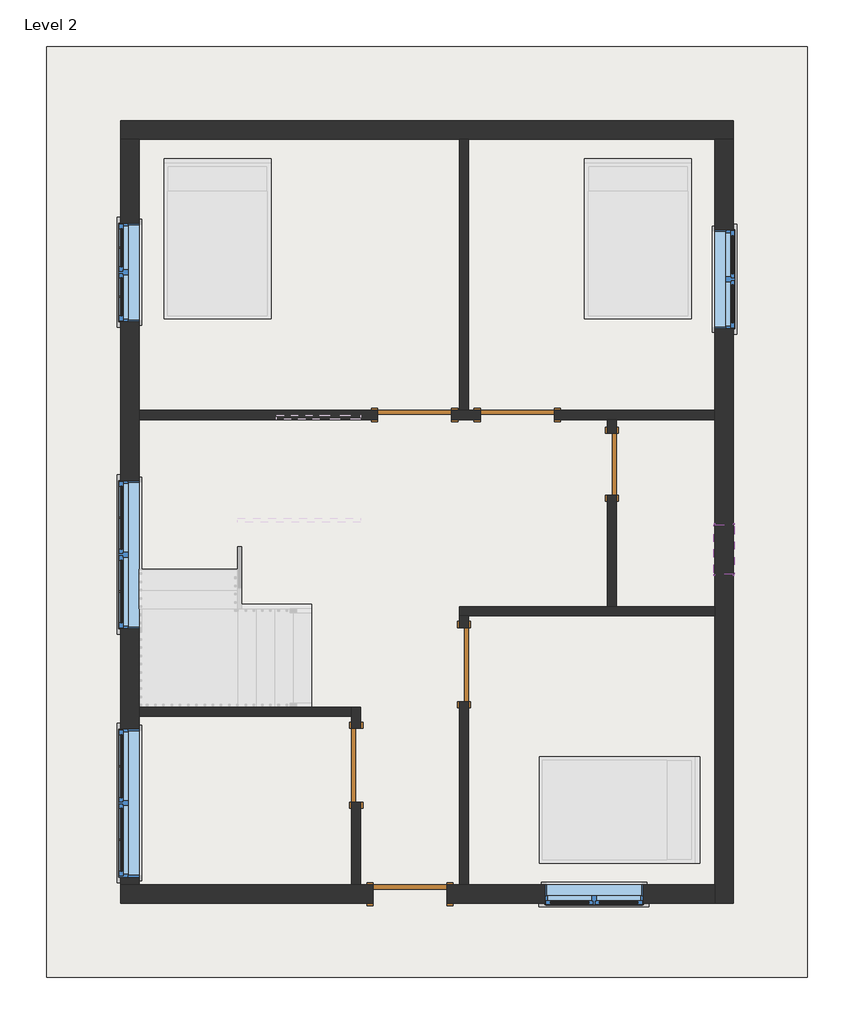
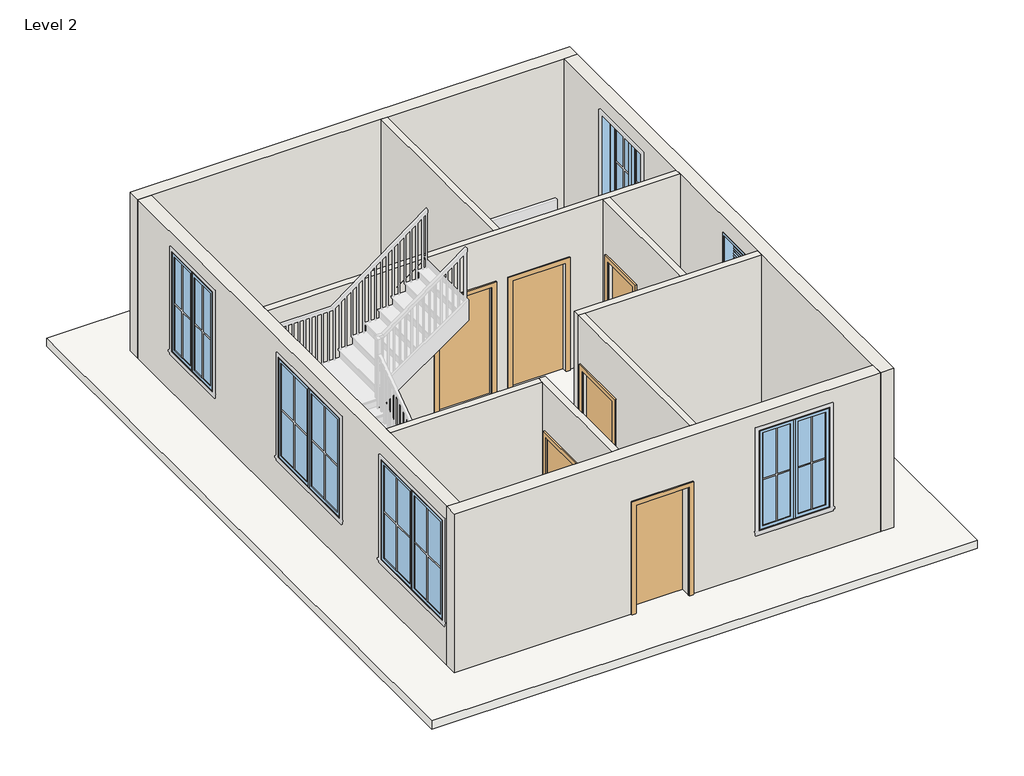
# One storey, part 1 of 3: 11 walls, 6 doors, 6 windows, 1 roof.
"""IFC4 building model written with IfcOpenShell, lengths in millimetres."""

from ifc_helpers import new_model, si_unit, frame, origin, place, context, project, spatial, polyline, outline, extrude, faceted_brep, transform, mapped, element, save
from components import door_f2b275c1, single_flush_door_3_e5f9f3c4, single_flush_door_3_305aa2a5, single_flush_door_3_a90ba1ad, window_casement_double_win_4_6ca1769e, window_casement_double_win_6_ce442eab, window_f2d8fef0

model = new_model("IFC4")

# Units and contexts
model_context = context("Model", 3, world=origin())
ifc_project = project(units=[si_unit("LENGTHUNIT", "METRE", prefix="MILLI")], contexts=[model_context])

# Site, building, storey
site = spatial("IfcSite", under=ifc_project)
building = spatial("IfcBuilding", under=site)
storey = spatial("IfcBuildingStorey", under=building, Name="Level 2", Elevation=3048.0)

# Doors
placement = place(None, origin())
door_shape = door_f2b275c1(model_context)
element("IfcDoor", 1, ObjectType="Single-Flush : 2'6\"", at=placement, inside=storey, context=model_context, shape_type="MappedRepresentation", body=[
    mapped(door_shape, transform((1031.6394609, 262.5126239, 3048.0), x_axis=(0.0, 1.0, 0.0), y_axis=(-1.0, 0.0, 0.0), z_axis=(0.0, 0.0, 1.0))),
])
single_flush_door_3_shape = single_flush_door_3_e5f9f3c4(model_context)
element("IfcDoor", 2, ObjectType="Single-Flush : door 3'", at=placement, inside=storey, context=model_context, shape_type="MappedRepresentation", body=[
    mapped(single_flush_door_3_shape, transform((-1406.7605391, 872.1126239, 3048.0), x_axis=(1.0, 0.0, 0.0), y_axis=(0.0, 1.0, 0.0), z_axis=(0.0, 0.0, 1.0))),
])
element("IfcDoor", 3, ObjectType="Single-Flush : door 3'", at=placement, inside=storey, context=model_context, shape_type="MappedRepresentation", body=[
    mapped(single_flush_door_3_shape, transform((-2130.6605391, -3458.5873761, 3048.0), x_axis=(0.0, 1.0, 0.0), y_axis=(-1.0, 0.0, 0.0), z_axis=(0.0, 0.0, 1.0))),
])
single_flush_door_3_2_shape = single_flush_door_3_305aa2a5(model_context)
element("IfcDoor", 4, ObjectType="Single-Flush : door 3'", at=placement, inside=storey, context=model_context, shape_type="MappedRepresentation", body=[
    mapped(single_flush_door_3_2_shape, transform((-136.7605391, 872.1126239, 3048.0), x_axis=(-1.0, 0.0, 0.0), y_axis=(0.0, -1.0, 0.0), z_axis=(0.0, 0.0, 1.0))),
])
element("IfcDoor", 5, ObjectType="Single-Flush : door 3'", at=placement, inside=storey, context=model_context, shape_type="MappedRepresentation", body=[
    mapped(single_flush_door_3_2_shape, transform((-797.1605391, -2213.9873761, 3048.0), x_axis=(0.0, 1.0, 0.0), y_axis=(-1.0, 0.0, 0.0), z_axis=(0.0, 0.0, 1.0))),
])
single_flush_door_3_3_shape = single_flush_door_3_a90ba1ad(model_context)
element("IfcDoor", 6, ObjectType="Single-Flush : door 3'", at=placement, inside=storey, context=model_context, shape_type="MappedRepresentation", body=[
    mapped(single_flush_door_3_3_shape, transform((-1463.9105391, -5052.4373761, 3048.0), x_axis=(-1.0, 0.0, 0.0), y_axis=(0.0, -1.0, 0.0), z_axis=(0.0, 0.0, 1.0))),
])

# Roof
element("IfcRoof", 7, ObjectType="Generic - 12\"", at=placement, inside=storey, context=model_context, shape_type="SweptSolid", body=[
    extrude(outline(polyline([(-5959.7105391, 5425.0626239), (3450.9894609, 5425.0626239), (3450.9894609, -6081.1373761), (-5959.7105391, -6081.1373761), (-5959.7105391, 5425.0626239)])), frame((0.0, 0.0, 3048.0), z_axis=(0.0, 0.0, 1.0), x_axis=(1.0, 0.0, 0.0)), (0.0, 0.0, 1.0), 152.4),
])

# Walls
element("IfcWall", 8, ObjectType="WALL 4.5\"", at=placement, inside=storey, context=model_context, shape_type="SweptSolid", body=[
    extrude(outline(polyline([(-854.3105391, 929.2626239), (-854.3105391, 4282.0626239), (-740.0105391, 4282.0626239), (-740.0105391, 929.2626239), (-854.3105391, 929.2626239)])), frame((0.0, 0.0, 3048.0), z_axis=(0.0, 0.0, 1.0), x_axis=(1.0, 0.0, 0.0)), (0.0, 0.0, 1.0), 3048.0),
])
element("IfcWall", 9, ObjectType="WALL 4.5\"", at=placement, inside=storey, context=model_context, shape_type="Brep", body=[
    faceted_brep([(-949.5605391, 814.9626239, 3048.0), (-593.9605391, 814.9626239, 3048.0), (-593.9605391, 814.9626239, 5181.6), (320.4394609, 814.9626239, 5181.6), (320.4394609, 814.9626239, 3048.0), (974.4894609, 814.9626239, 3048.0), (1088.7894609, 814.9626239, 3048.0), (2307.9894609, 814.9626239, 3048.0), (2307.9894609, 814.9626239, 6096.0), (1088.7894609, 814.9626239, 6096.0), (974.4894609, 814.9626239, 6096.0), (-4816.7105391, 814.9626239, 6096.0), (-4816.7105391, 814.9626239, 3048.0), (-1863.9605391, 814.9626239, 3048.0), (-1863.9605391, 814.9626239, 5181.6), (-949.5605391, 814.9626239, 5181.6), (-593.9605391, 929.2626239, 5181.6), (-593.9605391, 929.2626239, 3048.0), (-740.0105391, 929.2626239, 3048.0), (-854.3105391, 929.2626239, 3048.0), (-949.5605391, 929.2626239, 3048.0), (-949.5605391, 929.2626239, 5181.6), (-1863.9605391, 929.2626239, 5181.6), (-1863.9605391, 929.2626239, 3048.0), (-4816.7105391, 929.2626239, 3048.0), (-4816.7105391, 929.2626239, 6096.0), (-854.3105391, 929.2626239, 6096.0), (-740.0105391, 929.2626239, 6096.0), (2307.9894609, 929.2626239, 6096.0), (2307.9894609, 929.2626239, 3048.0), (320.4394609, 929.2626239, 3048.0), (320.4394609, 929.2626239, 5181.6)], [[[0, 1, 2, 3, 4, 5, 6, 7, 8, 9, 10, 11, 12, 13, 14, 15]], [[16, 17, 18, 19, 20, 21, 22, 23, 24, 25, 26, 27, 28, 29, 30, 31]], [[13, 12, 24, 23]], [[30, 29, 7, 6, 5, 4]], [[20, 19, 18, 17, 1, 0]], [[8, 7, 29, 28]], [[12, 11, 25, 24]], [[21, 20, 0, 15]], [[22, 21, 15, 14]], [[23, 22, 14, 13]], [[2, 1, 17, 16]], [[3, 2, 16, 31]], [[4, 3, 31, 30]], [[11, 10, 9, 8, 28, 27, 26, 25]]]),
])
element("IfcWall", 10, ObjectType="WALL 4.5\"", at=placement, inside=storey, context=model_context, shape_type="SweptSolid", body=[
    extrude(outline(polyline([(814.9626239, 3048.0), (643.5126239, 3048.0), (643.5126239, 5080.0), (-118.4873761, 5080.0), (-118.4873761, 3048.0), (-1496.4373761, 3048.0), (-1496.4373761, 6096.0), (814.9626239, 6096.0), (814.9626239, 3048.0)])), frame((974.4894609, 0.0, 0.0), z_axis=(1.0, 0.0, 0.0), x_axis=(0.0, 1.0, 0.0)), (0.0, 0.0, 1.0), 114.3),
])
element("IfcWall", 11, ObjectType="WALL 4.5\"", at=placement, inside=storey, context=model_context, shape_type="Brep", body=[
    faceted_brep([(2307.9894609, -1496.4373761, 3048.0), (1088.7894609, -1496.4373761, 3048.0), (974.4894609, -1496.4373761, 3048.0), (-854.3105391, -1496.4373761, 3048.0), (-854.3105391, -1496.4373761, 6096.0), (974.4894609, -1496.4373761, 6096.0), (1088.7894609, -1496.4373761, 6096.0), (2307.9894609, -1496.4373761, 6096.0), (2307.9894609, -1610.7373761, 3048.0), (2307.9894609, -1610.7373761, 6096.0), (-740.0105391, -1610.7373761, 6096.0), (-854.3105391, -1610.7373761, 6096.0), (-854.3105391, -1610.7373761, 3048.0), (-740.0105391, -1610.7373761, 3048.0)], [[[0, 1, 2, 3, 4, 5, 6, 7]], [[8, 9, 10, 11, 12, 13]], [[3, 2, 1, 0, 8, 13, 12]], [[0, 7, 9, 8]], [[4, 3, 12, 11]], [[7, 6, 5, 4, 11, 10, 9]]]),
])
element("IfcWall", 12, ObjectType="WALL 4.5\"", at=placement, inside=storey, context=model_context, shape_type="SweptSolid", body=[
    extrude(outline(polyline([(-1610.7373761, 3048.0), (-1756.7873761, 3048.0), (-1756.7873761, 5181.6), (-2671.1873761, 5181.6), (-2671.1873761, 3048.0), (-4938.1373761, 3048.0), (-4938.1373761, 6096.0), (-1610.7373761, 6096.0), (-1610.7373761, 3048.0)])), frame((-854.3105391, 0.0, 0.0), z_axis=(1.0, 0.0, 0.0), x_axis=(0.0, 1.0, 0.0)), (0.0, 0.0, 1.0), 114.3),
])
element("IfcWall", 13, ObjectType="WALL 4.5\"", at=placement, inside=storey, context=model_context, shape_type="Brep", body=[
    faceted_brep([(-2073.5105391, -3001.3873761, 5181.6), (-2073.5105391, -3001.3873761, 3048.0), (-2073.5105391, -2741.0373761, 3048.0), (-2073.5105391, -2741.0373761, 6096.0), (-2073.5105391, -4938.1373761, 6096.0), (-2073.5105391, -4938.1373761, 3048.0), (-2073.5105391, -3915.7873761, 3048.0), (-2073.5105391, -3915.7873761, 5181.6), (-2187.8105391, -2741.0373761, 3048.0), (-2187.8105391, -2855.3373761, 3048.0), (-2187.8105391, -3001.3873761, 3048.0), (-2187.8105391, -3001.3873761, 5181.6), (-2187.8105391, -3915.7873761, 5181.6), (-2187.8105391, -3915.7873761, 3048.0), (-2187.8105391, -4938.1373761, 3048.0), (-2187.8105391, -4938.1373761, 6096.0), (-2187.8105391, -2855.3373761, 6096.0), (-2187.8105391, -2741.0373761, 6096.0)], [[[0, 1, 2, 3, 4, 5, 6, 7]], [[8, 9, 10, 11, 12, 13, 14, 15, 16, 17]], [[6, 5, 14, 13]], [[2, 1, 10, 9, 8]], [[5, 4, 15, 14]], [[3, 2, 8, 17]], [[11, 10, 1, 0]], [[12, 11, 0, 7]], [[13, 12, 7, 6]], [[4, 3, 17, 16, 15]]]),
])
element("IfcWall", 14, ObjectType="WALL 4.5\"", at=placement, inside=storey, context=model_context, shape_type="SweptSolid", body=[
    extrude(outline(polyline([(-4816.7105391, -2741.0373761), (-2187.8105391, -2741.0373761), (-2187.8105391, -2855.3373761), (-4816.7105391, -2855.3373761), (-4816.7105391, -2741.0373761)])), frame((0.0, 0.0, 3048.0), z_axis=(0.0, 0.0, 1.0), x_axis=(1.0, 0.0, 0.0)), (0.0, 0.0, 1.0), 3048.0),
])
element("IfcWall", 15, ObjectType="WALL 9\"", at=placement, inside=storey, context=model_context, shape_type="Brep", body=[
    faceted_brep([(-5045.3105391, 4282.0626239, 3048.0), (-4816.7105391, 4282.0626239, 3048.0), (-854.3105391, 4282.0626239, 3048.0), (-740.0105391, 4282.0626239, 3048.0), (2307.9894609, 4282.0626239, 3048.0), (2536.5894609, 4282.0626239, 3048.0), (2536.5894609, 4282.0626239, 6096.0), (2307.9894609, 4282.0626239, 6096.0), (-740.0105391, 4282.0626239, 6096.0), (-854.3105391, 4282.0626239, 6096.0), (-4816.7105391, 4282.0626239, 6096.0), (-5045.3105391, 4282.0626239, 6096.0), (-5045.3105391, 4510.6626239, 3048.0), (-5045.3105391, 4510.6626239, 6096.0), (2536.5894609, 4510.6626239, 6096.0), (2536.5894609, 4510.6626239, 3048.0)], [[[0, 1, 2, 3, 4, 5, 6, 7, 8, 9, 10, 11]], [[12, 13, 14, 15]], [[5, 4, 3, 2, 1, 0, 12, 15]], [[6, 5, 15, 14]], [[0, 11, 13, 12]], [[11, 10, 9, 8, 7, 6, 14, 13]]]),
])
element("IfcWall", 16, ObjectType="WALL 9\"", at=placement, inside=storey, context=model_context, shape_type="Brep", body=[
    faceted_brep([(2307.9894609, 4282.0626239, 3048.0), (2307.9894609, 929.2626239, 3048.0), (2307.9894609, 814.9626239, 3048.0), (2307.9894609, -1496.4373761, 3048.0), (2307.9894609, -1610.7373761, 3048.0), (2307.9894609, -4938.1373761, 3048.0), (2307.9894609, -5166.7373761, 3048.0), (2307.9894609, -5166.7373761, 6096.0), (2307.9894609, -4938.1373761, 6096.0), (2307.9894609, -1610.7373761, 6096.0), (2307.9894609, -1496.4373761, 6096.0), (2307.9894609, 814.9626239, 6096.0), (2307.9894609, 929.2626239, 6096.0), (2307.9894609, 4282.0626239, 6096.0), (2307.9894609, 1938.9126239, 5791.2), (2307.9894609, 1938.9126239, 3962.4), (2307.9894609, 3158.1126239, 3962.4), (2307.9894609, 3158.1126239, 5791.2), (2307.9894609, -486.7873761, 5791.2), (2307.9894609, -1096.3873761, 5791.2), (2307.9894609, -1096.3873761, 5181.6), (2307.9894609, -486.7873761, 5181.6), (2536.5894609, 4282.0626239, 3048.0), (2536.5894609, 4282.0626239, 6096.0), (2536.5894609, -5166.7373761, 6096.0), (2536.5894609, -5166.7373761, 3048.0), (2536.5894609, 1938.9126239, 5791.2), (2536.5894609, 3158.1126239, 5791.2), (2536.5894609, 3158.1126239, 3962.4), (2536.5894609, 1938.9126239, 3962.4), (2536.5894609, -486.7873761, 5791.2), (2536.5894609, -486.7873761, 5181.6), (2536.5894609, -1096.3873761, 5181.6), (2536.5894609, -1096.3873761, 5791.2)], [[[0, 1, 2, 3, 4, 5, 6, 7, 8, 9, 10, 11, 12, 13], [14, 15, 16, 17], [18, 19, 20, 21]], [[22, 23, 24, 25], [26, 27, 28, 29], [30, 31, 32, 33]], [[6, 5, 4, 3, 2, 1, 0, 22, 25]], [[0, 13, 23, 22]], [[7, 6, 25, 24]], [[15, 14, 26, 29]], [[16, 15, 29, 28]], [[17, 16, 28, 27]], [[14, 17, 27, 26]], [[31, 30, 18, 21]], [[32, 31, 21, 20]], [[33, 32, 20, 19]], [[30, 33, 19, 18]], [[13, 12, 11, 10, 9, 8, 7, 24, 23]]]),
])
element("IfcWall", 17, ObjectType="WALL 9\"", at=placement, inside=storey, context=model_context, shape_type="Brep", body=[
    faceted_brep([(-1921.1105391, -4938.1373761, 5181.6), (-1921.1105391, -4938.1373761, 3048.0), (-2073.5105391, -4938.1373761, 3048.0), (-2187.8105391, -4938.1373761, 3048.0), (-4816.7105391, -4938.1373761, 3048.0), (-5045.3105391, -4938.1373761, 3048.0), (-5045.3105391, -4938.1373761, 6096.0), (-4816.7105391, -4938.1373761, 6096.0), (-2187.8105391, -4938.1373761, 6096.0), (-2073.5105391, -4938.1373761, 6096.0), (-854.3105391, -4938.1373761, 6096.0), (-740.0105391, -4938.1373761, 6096.0), (2307.9894609, -4938.1373761, 6096.0), (2307.9894609, -4938.1373761, 3048.0), (-740.0105391, -4938.1373761, 3048.0), (-854.3105391, -4938.1373761, 3048.0), (-1006.7105391, -4938.1373761, 3048.0), (-1006.7105391, -4938.1373761, 5181.6), (202.9644609, -4938.1373761, 5791.2), (202.9644609, -4938.1373761, 3962.4), (1422.1644609, -4938.1373761, 3962.4), (1422.1644609, -4938.1373761, 5791.2), (-5045.3105391, -5166.7373761, 3048.0), (-1921.1105391, -5166.7373761, 3048.0), (-1921.1105391, -5166.7373761, 5181.6), (-1006.7105391, -5166.7373761, 5181.6), (-1006.7105391, -5166.7373761, 3048.0), (2307.9894609, -5166.7373761, 3048.0), (2307.9894609, -5166.7373761, 6096.0), (-5045.3105391, -5166.7373761, 6096.0), (202.9644609, -5166.7373761, 5791.2), (1422.1644609, -5166.7373761, 5791.2), (1422.1644609, -5166.7373761, 3962.4), (202.9644609, -5166.7373761, 3962.4)], [[[0, 1, 2, 3, 4, 5, 6, 7, 8, 9, 10, 11, 12, 13, 14, 15, 16, 17], [18, 19, 20, 21]], [[22, 23, 24, 25, 26, 27, 28, 29], [30, 31, 32, 33]], [[5, 4, 3, 2, 1, 23, 22]], [[16, 15, 14, 13, 27, 26]], [[13, 12, 28, 27]], [[6, 5, 22, 29]], [[19, 18, 30, 33]], [[20, 19, 33, 32]], [[21, 20, 32, 31]], [[18, 21, 31, 30]], [[24, 23, 1, 0]], [[25, 24, 0, 17]], [[26, 25, 17, 16]], [[12, 11, 10, 9, 8, 7, 6, 29, 28]]]),
])
element("IfcWall", 18, ObjectType="WALL 9\"", at=placement, inside=storey, context=model_context, shape_type="Brep", body=[
    faceted_brep([(-4816.7105391, -4938.1373761, 3048.0), (-4816.7105391, -2855.3373761, 3048.0), (-4816.7105391, -2741.0373761, 3048.0), (-4816.7105391, 814.9626239, 3048.0), (-4816.7105391, 929.2626239, 3048.0), (-4816.7105391, 4282.0626239, 3048.0), (-4816.7105391, 4282.0626239, 6096.0), (-4816.7105391, 929.2626239, 6096.0), (-4816.7105391, 814.9626239, 6096.0), (-4816.7105391, -2741.0373761, 6096.0), (-4816.7105391, -2855.3373761, 6096.0), (-4816.7105391, -4938.1373761, 6096.0), (-4816.7105391, -3010.9123761, 5791.2), (-4816.7105391, -3010.9123761, 3962.4), (-4816.7105391, -4839.7123761, 3962.4), (-4816.7105391, -4839.7123761, 5791.2), (-4816.7105391, 59.3126239, 5791.2), (-4816.7105391, 59.3126239, 3962.4), (-4816.7105391, -1769.4873761, 3962.4), (-4816.7105391, -1769.4873761, 5791.2), (-4816.7105391, 3243.8376239, 5791.2), (-4816.7105391, 3243.8376239, 3962.4), (-4816.7105391, 2024.6376239, 3962.4), (-4816.7105391, 2024.6376239, 5791.2), (-5045.3105391, -4938.1373761, 3048.0), (-5045.3105391, -4938.1373761, 6096.0), (-5045.3105391, 4282.0626239, 6096.0), (-5045.3105391, 4282.0626239, 3048.0), (-5045.3105391, -3010.9123761, 5791.2), (-5045.3105391, -4839.7123761, 5791.2), (-5045.3105391, -4839.7123761, 3962.4), (-5045.3105391, -3010.9123761, 3962.4), (-5045.3105391, 59.3126239, 5791.2), (-5045.3105391, -1769.4873761, 5791.2), (-5045.3105391, -1769.4873761, 3962.4), (-5045.3105391, 59.3126239, 3962.4), (-5045.3105391, 3243.8376239, 5791.2), (-5045.3105391, 2024.6376239, 5791.2), (-5045.3105391, 2024.6376239, 3962.4), (-5045.3105391, 3243.8376239, 3962.4)], [[[0, 1, 2, 3, 4, 5, 6, 7, 8, 9, 10, 11], [12, 13, 14, 15], [16, 17, 18, 19], [20, 21, 22, 23]], [[24, 25, 26, 27], [28, 29, 30, 31], [32, 33, 34, 35], [36, 37, 38, 39]], [[5, 4, 3, 2, 1, 0, 24, 27]], [[6, 5, 27, 26]], [[0, 11, 25, 24]], [[13, 12, 28, 31]], [[14, 13, 31, 30]], [[15, 14, 30, 29]], [[12, 15, 29, 28]], [[17, 16, 32, 35]], [[18, 17, 35, 34]], [[19, 18, 34, 33]], [[16, 19, 33, 32]], [[21, 20, 36, 39]], [[22, 21, 39, 38]], [[23, 22, 38, 37]], [[20, 23, 37, 36]], [[11, 10, 9, 8, 7, 6, 26, 25]]]),
])

# Windows
window_casement_double_win_4_shape = window_casement_double_win_4_6ca1769e(model_context)
element("IfcWindow", 19, ObjectType="Window-Casement-Double : win 4'", at=placement, inside=storey, context=model_context, shape_type="MappedRepresentation", body=[
    mapped(window_casement_double_win_4_shape, transform((812.5644609, -5052.4373761, 3048.0), x_axis=(-1.0, 0.0, 0.0), y_axis=(0.0, -1.0, 0.0), z_axis=(0.0, 0.0, 1.0))),
])
element("IfcWindow", 20, ObjectType="Window-Casement-Double : win 4'", at=placement, inside=storey, context=model_context, shape_type="MappedRepresentation", body=[
    mapped(window_casement_double_win_4_shape, transform((2422.2894609, 2548.5126239, 3048.0), x_axis=(0.0, -1.0, 0.0), y_axis=(1.0, 0.0, 0.0), z_axis=(0.0, 0.0, 1.0))),
])
element("IfcWindow", 21, ObjectType="Window-Casement-Double : win 4'", at=placement, inside=storey, context=model_context, shape_type="MappedRepresentation", body=[
    mapped(window_casement_double_win_4_shape, transform((-4931.0105391, 2634.2376239, 3048.0), x_axis=(0.0, 1.0, 0.0), y_axis=(-1.0, 0.0, 0.0), z_axis=(0.0, 0.0, 1.0))),
])
window_casement_double_win_6_shape = window_casement_double_win_6_ce442eab(model_context)
element("IfcWindow", 22, ObjectType="Window-Casement-Double : win 6'", at=placement, inside=storey, context=model_context, shape_type="MappedRepresentation", body=[
    mapped(window_casement_double_win_6_shape, transform((-4931.0105391, -3925.3123761, 3048.0), x_axis=(0.0, 1.0, 0.0), y_axis=(-1.0, 0.0, 0.0), z_axis=(0.0, 0.0, 1.0))),
])
element("IfcWindow", 23, ObjectType="Window-Casement-Double : win 6'", at=placement, inside=storey, context=model_context, shape_type="MappedRepresentation", body=[
    mapped(window_casement_double_win_6_shape, transform((-4931.0105391, -855.0873761, 3048.0), x_axis=(0.0, 1.0, 0.0), y_axis=(-1.0, 0.0, 0.0), z_axis=(0.0, 0.0, 1.0))),
])
window_shape = window_f2d8fef0(model_context)
element("IfcWindow", 24, ObjectType="Window-Louvers : 24\" x 24\"", at=placement, inside=storey, context=model_context, shape_type="MappedRepresentation", body=[
    mapped(window_shape, transform((2428.6394609, -791.5873761, 4267.2), x_axis=(0.0, -1.0, 0.0), y_axis=(1.0, 0.0, 0.0), z_axis=(0.0, 0.0, 1.0))),
])

save(model, "model.ifc")

# Revit data of these elements
# Type "Single-Flush : 2'6\""
#   Type Mark = "9"
#   Construction Type Id = "MDOOR"
#   Assembly Code = "C1020"
#   Analytic Construction = "Metal"
#   Thickness = 0' - 2"
#   Heat Transfer Coefficient (U) = 0.651978 BTU/(h·ft²·°F)
#   Height = 6' - 8"
#   Trim Projection Ext = 0' - 1"
#   Trim Projection Int = 0' - 1"
#   Trim Width = 0' - 3"
#   Width = 2' - 6"
#   Define Thermal Properties by = 1
#   Door Material = Door - Panel
#   Frame Material = Door - Frame
#   Visual Light Transmittance = 0
#   Solar Heat Gain Coefficient = 0
#   Function = (empty or 0)
#   Wall Closure = (empty or 0)
# Type "Single-Flush : door 3'"
#   Type Mark = "8"
#   Construction Type Id = "MDOOR"
#   Assembly Code = "C1020"
#   Analytic Construction = "Metal"
#   Thickness = 0' - 2"
#   Heat Transfer Coefficient (U) = 0.651978 BTU/(h·ft²·°F)
#   Height = 7' - 0"
#   Trim Projection Ext = 0' - 1"
#   Trim Projection Int = 0' - 1"
#   Trim Width = 0' - 3"
#   Width = 3' - 0"
#   Define Thermal Properties by = 1
#   Door Material = Door - Panel
#   Frame Material = Door - Frame
#   Visual Light Transmittance = 0
#   Solar Heat Gain Coefficient = 0
#   Function = (empty or 0)
#   Wall Closure = (empty or 0)
# Type "Generic - 12\""
#   Assembly Code = "B1020"
#   Layers, outside or top first: 0' - 6" no material (function 1)
# Type "WALL 4.5\""
#   Assembly Code = "B2010"
#   Layers, outside or top first: 0' - 4 1/2" no material (function 1)
# Type "WALL 9\""
#   Assembly Code = "B2010"
#   Layers, outside or top first: 0' - 9" no material (function 1)
# Type "Window-Casement-Double : win 4'"
#   Type Mark = "19"
#   Fire Rating = "0.5h"
#   Assembly Code = "B2020100"
#   Analytic Construction = "Double glazing - domestic"
#   Frame Extension [instance default] = 0' - 0 1/4"
#   Window Inset [instance default] = 0' - 0"
#   Wall Thickness [instance default] = 0' - 6"
#   Interior Wall Closure [instance default] = 0' - 2 1/4"
#   Half Width = 2' - 0"
#   Visual Light Transmittance = 0.81
#   Thermal Resistance (R) = 1.8146 (h·ft²·°F)/BTU
#   Solar Heat Gain Coefficient = 0.76
#   Rough Width = 4' - 0 1/2"
#   Rough Height = 6' - 0 1/2"
#   Height = 6' - 0"
#   Heat Transfer Coefficient (U) = 0.5511 BTU/(h·ft²·°F)
#   Exterior Wall Closure [instance default] = 0' - 1 1/4"
#   Extension Jamb [instance default] = 0' - 2 1/4"
#   Default Sill Height = 3' - 0"
#   Width = 4' - 0"
#   Muntin Visibility = yes
#   Interior Trim Visibility [instance default] = yes
#   Exterior Trim Visibility [instance default] = yes
#   Extension Jamb Visibility [instance default] = yes
#   Interior Trim Material = Wood - Stained
#   Muntin Pattern = Muntin Pattern_2x2 : Muntin Pattern_2x2
#   Interior Trim = Trim-Window-Interior-Flat : Picture Frame
#   Interior Frame Material = Wood - Stained
#   Glass Panel Material = Glass
#   Exterior Trim Material = Clad - White
#   Exterior Trim = Trim-Window-Exterior-Flat : with Sill
#   Exterior Frame Material = Clad - White
#   Wall Closure = (empty or 0)
# Type "Window-Casement-Double : win 6'"
#   Type Mark = "18"
#   Fire Rating = "0.5h"
#   Assembly Code = "B2020100"
#   Analytic Construction = "Double glazing - domestic"
#   Frame Extension [instance default] = 0' - 0 1/4"
#   Window Inset [instance default] = 0' - 0"
#   Wall Thickness [instance default] = 0' - 6"
#   Interior Wall Closure [instance default] = 0' - 2 1/4"
#   Half Width = 3' - 0"
#   Visual Light Transmittance = 0.81
#   Thermal Resistance (R) = 1.8146 (h·ft²·°F)/BTU
#   Solar Heat Gain Coefficient = 0.76
#   Rough Width = 6' - 0 1/2"
#   Rough Height = 6' - 0 1/2"
#   Height = 6' - 0"
#   Heat Transfer Coefficient (U) = 0.5511 BTU/(h·ft²·°F)
#   Exterior Wall Closure [instance default] = 0' - 1 1/4"
#   Extension Jamb [instance default] = 0' - 2 1/4"
#   Default Sill Height = 3' - 0"
#   Width = 6' - 0"
#   Muntin Visibility = yes
#   Interior Trim Visibility [instance default] = yes
#   Exterior Trim Visibility [instance default] = yes
#   Extension Jamb Visibility [instance default] = yes
#   Interior Trim Material = Wood - Stained
#   Muntin Pattern = Muntin Pattern_2x2 : Muntin Pattern_2x2
#   Interior Trim = Trim-Window-Interior-Flat : Picture Frame
#   Interior Frame Material = Wood - Stained
#   Glass Panel Material = Glass
#   Exterior Trim Material = Clad - White
#   Exterior Trim = Trim-Window-Exterior-Flat : with Sill
#   Exterior Frame Material = Clad - White
#   Wall Closure = (empty or 0)
# Type "Window-Louvers : 24\" x 24\""
#   Type Mark = "20"
#   Construction Type Id = "GSP4R"
#   Assembly Code = "B20"
#   Analytic Construction = "1/8 in Pilkington single glazing"
#   Visual Light Transmittance = 0.9
#   Thermal Resistance (R) = 1.53941 (h·ft²·°F)/BTU
#   Solar Heat Gain Coefficient = 0.78
#   Max Height = 1' - 11.74264"
#   Height = 2' - 0"
#   Heat Transfer Coefficient (U) = 0.6496 BTU/(h·ft²·°F)
#   Blade Width [instance default] = 1' - 10 1/2"
#   Blade Vertical Thickness = 0' - 0.35355"
#   Blade Thickness = 0' - 0 1/4"
#   Blade Spacing = 0' - 1 1/2"
#   Blade Height = 0' - 1.85355"
#   Blade Depth = 0' - 3"
#   Blade Angle = 45.00°
#   Default Sill Height = 3' - 0"
#   Trim Projection_Exterior = 0' - 0 1/2"
#   Trim Projection_Interior = 0' - 0 1/2"
#   Trim Width_Exterior = 0' - 1 1/2"
#   Trim Width_Interior = 0' - 1 1/2"
#   Width = 2' - 0"
#   Max Blade Count = 12
#   Define Thermal Properties by = 1
#   Blade Count = 12
#   Frame Material = Birch
#   Louver Material = Birch
#   Trim Exterior Material = Birch
#   Trim Interior Material = Birch
#   Wall Closure = (empty or 0)
# Element 1 (IfcDoor, "Single-Flush : 2'6\"")
#   Phase Created = New Construction
#   Materials on its faces: "Door - Frame", "Door - Panel"
# Elements 2, 3, 4, 5, 6 (IfcDoor, "Single-Flush : door 3'")
#   Phase Created = New Construction
#   Materials on its faces: "Door - Frame", "Door - Panel"
# Element 7 (IfcRoof, "Generic - 12\"")
#   built-in parameter 1001705 = 10.5 (stored number, unit not read)
#   built-in parameter 1001710 = 33615
#   Phase Created = New Construction
#   Materials on its faces: "Wood Planks", "Wood - Stained"
# Elements 8, 9, 10, 11, 12, 13, 14 (IfcWall, "WALL 4.5\"")
#   Top Offset = 0' - 0"
#   Base Offset = 0' - 0"
#   Unconnected Height = 10' - 0"
#   wall height = 10' - 0"
#   Phase Created = New Construction
#   Base Constraint = Level 2
#   Materials on its faces: "Default Wall"
# Elements 15, 16, 17, 18 (IfcWall, "WALL 9\"")
#   Top Offset = 0' - 0"
#   Base Offset = 0' - 0"
#   Unconnected Height = 10' - 0"
#   wall height = 10' - 0"
#   Phase Created = New Construction
#   Base Constraint = Level 2
#   Materials on its faces: "Default Wall", "Door - Frame"
# Element 19 (IfcWindow, "Window-Casement-Double : win 4'")
#   Mark = "9"
#   Window Inset = 0' - 0"
#   Interior Wall Closure = 0' - 2 1/4"
#   Frame Extension = 0' - 0 1/4"
#   Exterior Wall Closure = 0' - 1 1/4"
#   Interior Trim Visibility = yes
#   Exterior Trim Visibility = yes
#   Phase Created = New Construction
#   Materials on its faces: "Wood - Stained", "Glass", "Clad - White"
# Element 20 (IfcWindow, "Window-Casement-Double : win 4'")
#   Mark = "10"
#   Window Inset = 0' - 0"
#   Interior Wall Closure = 0' - 2 1/4"
#   Frame Extension = 0' - 0 1/4"
#   Exterior Wall Closure = 0' - 1 1/4"
#   Interior Trim Visibility = yes
#   Exterior Trim Visibility = yes
#   Phase Created = New Construction
#   Materials on its faces: "Wood - Stained", "Glass", "Clad - White"
# Element 21 (IfcWindow, "Window-Casement-Double : win 4'")
#   Mark = "11"
#   Window Inset = 0' - 0"
#   Interior Wall Closure = 0' - 2 1/4"
#   Frame Extension = 0' - 0 1/4"
#   Exterior Wall Closure = 0' - 1 1/4"
#   Interior Trim Visibility = yes
#   Exterior Trim Visibility = yes
#   Phase Created = New Construction
#   Materials on its faces: "Wood - Stained", "Glass", "Clad - White"
# Element 22 (IfcWindow, "Window-Casement-Double : win 6'")
#   Mark = "7"
#   Window Inset = 0' - 0"
#   Interior Wall Closure = 0' - 2 1/4"
#   Frame Extension = 0' - 0 1/4"
#   Exterior Wall Closure = 0' - 1 1/4"
#   Interior Trim Visibility = yes
#   Exterior Trim Visibility = yes
#   Phase Created = New Construction
#   Materials on its faces: "Wood - Stained", "Glass", "Clad - White"
# Element 23 (IfcWindow, "Window-Casement-Double : win 6'")
#   Mark = "8"
#   Window Inset = 0' - 0"
#   Interior Wall Closure = 0' - 2 1/4"
#   Frame Extension = 0' - 0 1/4"
#   Exterior Wall Closure = 0' - 1 1/4"
#   Interior Trim Visibility = yes
#   Exterior Trim Visibility = yes
#   Phase Created = New Construction
#   Materials on its faces: "Wood - Stained", "Glass", "Clad - White"
# Element 24 (IfcWindow, "Window-Louvers : 24\" x 24\"")
#   Mark = "12"
#   Blade Width = 1' - 10 1/2"
#   Phase Created = New Construction
#   Materials on its faces: "Birch"
# Materials
#   "Door - Panel": class "Wood", colour RGB 210 159 95, transparency 0, Cost = 0
#   "Door - Frame": colour RGB 118 70 51, transparency 0, Cost = 0
#   "Wood - Stained": class "Wood", colour RGB 224 178 126, transparency 0, Cost = 0
#   "Glass": class "Glass", colour RGB 0 128 192, transparency 0.75, Description = "Soda Lime Glass", Cost = 0
#   "Clad - White": class "Wood", colour RGB 242 242 238, transparency 0, Cost = 0
#   "Birch": class "Wood", colour RGB 224 178 126, transparency 0, Description = "Betula Alleghaniensis", Cost = 0
#   "Wood Planks": class "Wood", colour RGB 193 160 115, transparency 0, Description = "Physical material.", Cost = 0
#   "Default Wall": colour RGB 128 128 128, transparency 0, Cost = 0
